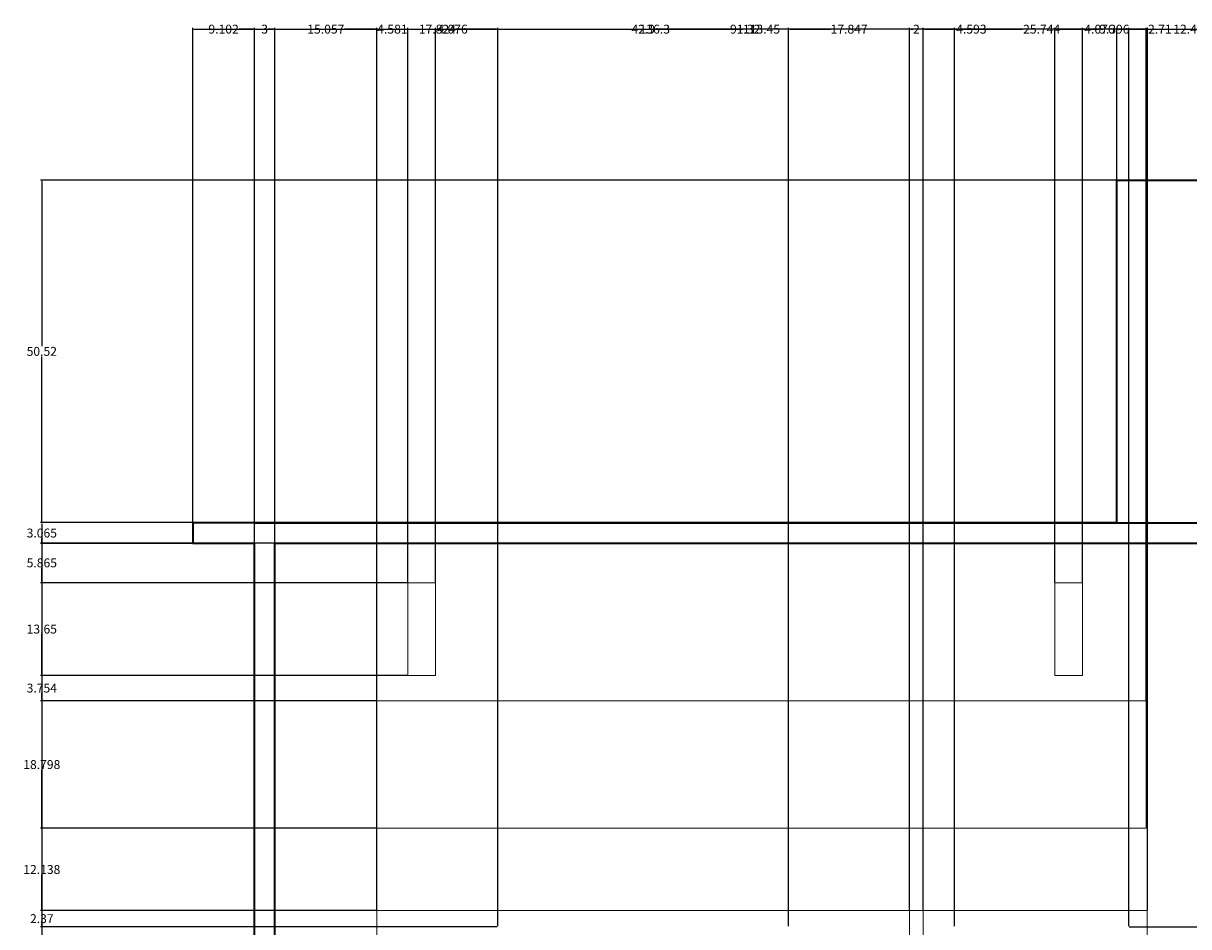
# Model space of a CAD drawing. Units: inches. Extents: x 30 to 515, y 94 to 489.
# Tile 3 of 7: x 30 to 202, y 356 to 489. Entities that reach past the tile are written whole.
import ezdxf

# ---------------------------------------------------------------- set-up
doc = ezdxf.new("R2010")
doc.units = ezdxf.units.IN
doc.header["$MEASUREMENT"] = 0
for name, color, linetype, lineweight in [('A-ANNO-DIMS', 2, 'Continuous', 18), ('A-ELEV', 8, 'Continuous', 18), ('A-FLOR-HRAL', 3, 'Continuous', 18), ('A-ROOF', 1, 'Continuous', 35), ('A-WALL', 7, 'Continuous', 35)]:
    doc.layers.add(name, color=color, linetype=linetype, lineweight=lineweight)
doc.styles.get("Standard").update_dxf_attribs({"font": 'arial.ttf'})
doc.dimstyles.get("Standard").update_dxf_attribs({"dimtxt": 1.3125, "dimasz": 0.18, "dimexe": 0.18, "dimexo": 0.0625, "dimgap": 0.09, "dimtad": 0, "dimtih": 1, "dimtoh": 1, "dimdec": 4, "dimzin": 0, "dimdsep": 46, "dimlunit": 4, "dimtxsty": 'Standard', "dimcen": 0.09, "dimadec": 0, "dimazin": 0, "dimtfac": 1, "dimtdec": 4, "dimtofl": 0, "dimtmove": 0, "dimatfit": 3, "dimfxl": 1, "dimtolj": 1, "dimtzin": 0, "dimarcsym": 0})

# ---------------------------------------------------------------- blocks, each defined once
blk = doc.blocks.new('*D4')
at = {"layer": 'A-ANNO-DIMS', "color": 0, "lineweight": -2, "transparency": 16777216}
for p, q in [((54.91, 415.59), (54.91, 488.48)), ((55.09, 488.3), (120.82, 488.3)), ((191.03, 488.3), (125.31, 488.3)), ((191.21, 466.11), (191.21, 488.48))]:
    blk.add_line(p, q, dxfattribs=at)
at = {"layer": 'A-ANNO-DIMS', "color": 0, "transparency": 16777216}
for points in [[(55.09, 488.33), (55.09, 488.27), (54.91, 488.3)], [(191.03, 488.33), (191.03, 488.27), (191.21, 488.3)]]:
    blk.add_solid(points, dxfattribs=at)
at = {"layer": 'Defpoints', "color": 0, "transparency": 16777216}
for p in [(191.21, 488.3), (191.21, 466.05), (54.91, 415.53)]:
    blk.add_point(p, dxfattribs=at)
at = {"layer": 'A-ANNO-DIMS', "color": 0, "transparency": 16777216, "insert": (123.06, 488.3), "char_height": 1.312, "attachment_point": 5}
blk.add_mtext('\\A1;136.3', dxfattribs=at)
blk = doc.blocks.new('*D5')
at = {"layer": 'A-ANNO-DIMS', "color": 0, "lineweight": -2, "transparency": 16777216}
for p, q in [((191.21, 466.11), (191.21, 488.48)), ((191.39, 488.3), (285.04, 488.3)), ((384.19, 488.3), (290.54, 488.3)), ((384.37, 466.11), (384.37, 488.48))]:
    blk.add_line(p, q, dxfattribs=at)
at = {"layer": 'A-ANNO-DIMS', "color": 0, "transparency": 16777216}
for points in [[(191.39, 488.33), (191.39, 488.27), (191.21, 488.3)], [(384.19, 488.33), (384.19, 488.27), (384.37, 488.3)]]:
    blk.add_solid(points, dxfattribs=at)
at = {"layer": 'Defpoints', "color": 0, "transparency": 16777216}
for p in [(384.37, 488.3), (191.21, 466.05), (384.37, 466.05)]:
    blk.add_point(p, dxfattribs=at)
at = {"layer": 'A-ANNO-DIMS', "color": 0, "transparency": 16777216, "insert": (287.79, 488.3), "char_height": 1.312, "attachment_point": 5}
blk.add_mtext('\\A1;193.16', dxfattribs=at)
blk = doc.blocks.new('*D25')
at = {"layer": 'A-ANNO-DIMS', "color": 0, "lineweight": -2, "transparency": 16777216}
for p, q in [((66.95, 415.53), (32.48, 415.53)), ((32.66, 415.35), (32.66, 342.78)), ((32.66, 268.71), (32.66, 341.28)), ((66.95, 268.53), (32.48, 268.53))]:
    blk.add_line(p, q, dxfattribs=at)
at = {"layer": 'A-ANNO-DIMS', "color": 0, "transparency": 16777216}
for points in [[(32.63, 415.35), (32.69, 415.35), (32.66, 415.53)], [(32.63, 268.71), (32.69, 268.71), (32.66, 268.53)]]:
    blk.add_solid(points, dxfattribs=at)
at = {"layer": 'Defpoints', "color": 0, "transparency": 16777216}
for p in [(32.66, 415.53), (67.02, 415.53), (67.02, 268.53)]:
    blk.add_point(p, dxfattribs=at)
at = {"layer": 'A-ANNO-DIMS', "color": 0, "transparency": 16777216, "insert": (32.66, 342.03), "char_height": 1.312, "attachment_point": 5}
blk.add_mtext('\\A1;147', dxfattribs=at)
blk = doc.blocks.new('*D26')
at = {"layer": 'A-ANNO-DIMS', "color": 0, "lineweight": -2, "transparency": 16777216}
for p, q in [((54.85, 415.53), (32.48, 415.53)), ((32.66, 415.35), (32.66, 414.76)), ((32.66, 412.64), (32.66, 413.23)), ((54.85, 412.46), (32.48, 412.46))]:
    blk.add_line(p, q, dxfattribs=at)
at = {"layer": 'A-ANNO-DIMS', "color": 0, "transparency": 16777216}
for points in [[(32.63, 415.35), (32.69, 415.35), (32.66, 415.53)], [(32.63, 412.64), (32.69, 412.64), (32.66, 412.46)]]:
    blk.add_solid(points, dxfattribs=at)
at = {"layer": 'Defpoints', "color": 0, "transparency": 16777216}
for p in [(32.66, 415.53), (54.91, 415.53), (54.91, 412.46)]:
    blk.add_point(p, dxfattribs=at)
at = {"layer": 'A-ANNO-DIMS', "color": 0, "transparency": 16777216, "insert": (32.66, 414), "char_height": 1.312, "attachment_point": 5}
blk.add_mtext('\\A1;3.065', dxfattribs=at)
blk = doc.blocks.new('*D27')
at = {"layer": 'A-ANNO-DIMS', "color": 0, "lineweight": -2, "transparency": 16777216}
for p, q in [((191.15, 466.05), (32.48, 466.05)), ((32.66, 465.87), (32.66, 441.55)), ((32.66, 415.71), (32.66, 440.03)), ((191.15, 415.53), (32.48, 415.53))]:
    blk.add_line(p, q, dxfattribs=at)
at = {"layer": 'A-ANNO-DIMS', "color": 0, "transparency": 16777216}
for points in [[(32.63, 465.87), (32.69, 465.87), (32.66, 466.05)], [(32.63, 415.71), (32.69, 415.71), (32.66, 415.53)]]:
    blk.add_solid(points, dxfattribs=at)
at = {"layer": 'Defpoints', "color": 0, "transparency": 16777216}
for p in [(32.66, 466.05), (191.21, 466.05), (191.21, 415.53)]:
    blk.add_point(p, dxfattribs=at)
at = {"layer": 'A-ANNO-DIMS', "color": 0, "transparency": 16777216, "insert": (32.66, 440.79), "char_height": 1.312, "attachment_point": 5}
blk.add_mtext('\\A1;50.52', dxfattribs=at)
blk = doc.blocks.new('*D31')
at = {"layer": 'A-ANNO-DIMS', "color": 0, "lineweight": -2, "transparency": 16777216}
for p, q in [((54.91, 412.53), (54.91, 488.48)), ((55.09, 488.3), (57.17, 488.3)), ((63.84, 488.3), (61.76, 488.3)), ((64.02, 412.57), (64.02, 488.48))]:
    blk.add_line(p, q, dxfattribs=at)
at = {"layer": 'A-ANNO-DIMS', "color": 0, "transparency": 16777216}
for points in [[(55.09, 488.33), (55.09, 488.27), (54.91, 488.3)], [(63.84, 488.33), (63.84, 488.27), (64.02, 488.3)]]:
    blk.add_solid(points, dxfattribs=at)
at = {"layer": 'Defpoints', "color": 0, "transparency": 16777216}
for p in [(64.02, 488.3), (64.02, 412.51), (54.91, 412.46)]:
    blk.add_point(p, dxfattribs=at)
at = {"layer": 'A-ANNO-DIMS', "color": 0, "transparency": 16777216, "insert": (59.47, 488.3), "char_height": 1.312, "attachment_point": 5}
blk.add_mtext('\\A1;9.102', dxfattribs=at)
blk = doc.blocks.new('*D32')
at = {"layer": 'A-ANNO-DIMS', "color": 0, "lineweight": -2, "transparency": 16777216}
for p, q in [((64.02, 412.57), (64.02, 488.48)), ((64.2, 488.3), (65, 488.3)), ((66.84, 488.3), (66.04, 488.3)), ((67.02, 412.59), (67.02, 488.48))]:
    blk.add_line(p, q, dxfattribs=at)
at = {"layer": 'A-ANNO-DIMS', "color": 0, "transparency": 16777216}
for points in [[(64.2, 488.33), (64.2, 488.27), (64.02, 488.3)], [(66.84, 488.33), (66.84, 488.27), (67.02, 488.3)]]:
    blk.add_solid(points, dxfattribs=at)
at = {"layer": 'Defpoints', "color": 0, "transparency": 16777216}
for p in [(67.02, 488.3), (64.02, 412.51), (67.02, 412.53)]:
    blk.add_point(p, dxfattribs=at)
at = {"layer": 'A-ANNO-DIMS', "color": 0, "transparency": 16777216, "insert": (65.52, 488.3), "char_height": 1.312, "attachment_point": 5}
blk.add_mtext('\\A1;3', dxfattribs=at)
blk = doc.blocks.new('*D33')
at = {"layer": 'A-ANNO-DIMS', "color": 0, "lineweight": -2, "transparency": 16777216}
for p, q in [((67.02, 412.59), (67.02, 488.48)), ((67.2, 488.3), (71.79, 488.3)), ((81.89, 488.3), (77.3, 488.3)), ((82.07, 389.32), (82.07, 488.48))]:
    blk.add_line(p, q, dxfattribs=at)
at = {"layer": 'A-ANNO-DIMS', "color": 0, "transparency": 16777216}
for points in [[(67.2, 488.33), (67.2, 488.27), (67.02, 488.3)], [(81.89, 488.33), (81.89, 488.27), (82.07, 488.3)]]:
    blk.add_solid(points, dxfattribs=at)
at = {"layer": 'Defpoints', "color": 0, "transparency": 16777216}
for p in [(82.07, 488.3), (67.02, 412.53), (82.07, 389.26)]:
    blk.add_point(p, dxfattribs=at)
at = {"layer": 'A-ANNO-DIMS', "color": 0, "transparency": 16777216, "insert": (74.55, 488.3), "char_height": 1.312, "attachment_point": 5}
blk.add_mtext('\\A1;15.057', dxfattribs=at)
blk = doc.blocks.new('*D34')
at = {"layer": 'A-ANNO-DIMS', "color": 0, "lineweight": -2, "transparency": 16777216}
for p, q in [((81.893567, 488.300291), (81.713567, 488.300291)), ((82.073567, 389.322756), (82.073567, 488.480291)), ((86.654989, 406.725431), (86.654989, 488.480291)), ((86.834989, 488.300291), (87.014989, 488.300291))]:
    blk.add_line(p, q, dxfattribs=at)
at = {"layer": 'A-ANNO-DIMS', "color": 0, "transparency": 16777216}
for points in [[(81.893567, 488.330291), (81.893567, 488.270291), (82.073567, 488.300291)], [(86.834989, 488.330291), (86.834989, 488.270291), (86.654989, 488.300291)]]:
    blk.add_solid(points, dxfattribs=at)
at = {"layer": 'Defpoints', "color": 0, "transparency": 16777216}
for p in [(86.654989, 488.300291), (86.654989, 406.662931), (82.073567, 389.260256)]:
    blk.add_point(p, dxfattribs=at)
at = {"layer": 'A-ANNO-DIMS', "color": 0, "transparency": 16777216, "insert": (84.364278, 488.300291), "char_height": 1.3125, "attachment_point": 5}
blk.add_mtext('\\A1;4.581', dxfattribs=at)
blk = doc.blocks.new('*D35')
at = {"layer": 'A-ANNO-DIMS', "color": 0, "lineweight": -2, "transparency": 16777216}
for p, q in [((86.65, 406.73), (86.65, 488.48)), ((86.83, 488.3), (90.55, 488.3)), ((90.73, 406.73), (90.73, 488.48)), ((90.73, 488.3), (90.91, 488.3))]:
    blk.add_line(p, q, dxfattribs=at)
at = {"layer": 'A-ANNO-DIMS', "color": 0, "transparency": 16777216}
for points in [[(86.83, 488.33), (86.83, 488.27), (86.65, 488.3)], [(90.55, 488.33), (90.55, 488.27), (90.73, 488.3)]]:
    blk.add_solid(points, dxfattribs=at)
at = {"layer": 'Defpoints', "color": 0, "transparency": 16777216}
for p in [(90.73, 488.3), (86.65, 406.66), (90.73, 406.66)]:
    blk.add_point(p, dxfattribs=at)
at = {"layer": 'A-ANNO-DIMS', "color": 0, "transparency": 16777216, "insert": (93.24, 488.3), "char_height": 1.312, "attachment_point": 5}
blk.add_mtext('\\A1;4.076', dxfattribs=at)
blk = doc.blocks.new('*D36')
at = {"layer": 'A-ANNO-DIMS', "color": 0, "lineweight": -2, "transparency": 16777216}
for p, q in [((90.73, 406.73), (90.73, 488.48)), ((90.91, 488.3), (134.09, 488.3)), ((181.87, 488.3), (138.69, 488.3)), ((182.05, 406.73), (182.05, 488.48))]:
    blk.add_line(p, q, dxfattribs=at)
at = {"layer": 'A-ANNO-DIMS', "color": 0, "transparency": 16777216}
for points in [[(90.91, 488.33), (90.91, 488.27), (90.73, 488.3)], [(181.87, 488.33), (181.87, 488.27), (182.05, 488.3)]]:
    blk.add_solid(points, dxfattribs=at)
at = {"layer": 'Defpoints', "color": 0, "transparency": 16777216}
for p in [(182.05, 488.3), (90.73, 406.66), (182.05, 406.66)]:
    blk.add_point(p, dxfattribs=at)
at = {"layer": 'A-ANNO-DIMS', "color": 0, "transparency": 16777216, "insert": (136.39, 488.3), "char_height": 1.312, "attachment_point": 5}
blk.add_mtext('\\A1;91.32', dxfattribs=at)
blk = doc.blocks.new('*D37')
at = {"layer": 'A-ANNO-DIMS', "color": 0, "lineweight": -2, "transparency": 16777216}
for p, q in [((182.05, 406.73), (182.05, 488.48)), ((182.23, 488.3), (185.95, 488.3)), ((186.13, 406.73), (186.13, 488.48)), ((186.13, 488.3), (186.31, 488.3))]:
    blk.add_line(p, q, dxfattribs=at)
at = {"layer": 'A-ANNO-DIMS', "color": 0, "transparency": 16777216}
for points in [[(182.23, 488.33), (182.23, 488.27), (182.05, 488.3)], [(185.95, 488.33), (185.95, 488.27), (186.13, 488.3)]]:
    blk.add_solid(points, dxfattribs=at)
at = {"layer": 'Defpoints', "color": 0, "transparency": 16777216}
for p in [(186.13, 488.3), (182.05, 406.66), (186.13, 406.66)]:
    blk.add_point(p, dxfattribs=at)
at = {"layer": 'A-ANNO-DIMS', "color": 0, "transparency": 16777216, "insert": (188.64, 488.3), "char_height": 1.312, "attachment_point": 5}
blk.add_mtext('\\A1;4.076', dxfattribs=at)
blk = doc.blocks.new('*D38')
at = {"layer": 'A-ANNO-DIMS', "color": 0, "lineweight": -2, "transparency": 16777216}
for p, q in [((186.13, 406.73), (186.13, 488.48)), ((186.31, 488.3), (188.52, 488.3)), ((195.35, 488.3), (193.13, 488.3)), ((195.53, 389.32), (195.53, 488.48))]:
    blk.add_line(p, q, dxfattribs=at)
at = {"layer": 'A-ANNO-DIMS', "color": 0, "transparency": 16777216}
for points in [[(186.31, 488.33), (186.31, 488.27), (186.13, 488.3)], [(195.35, 488.33), (195.35, 488.27), (195.53, 488.3)]]:
    blk.add_solid(points, dxfattribs=at)
at = {"layer": 'Defpoints', "color": 0, "transparency": 16777216}
for p in [(195.53, 488.3), (186.13, 406.66), (195.53, 389.26)]:
    blk.add_point(p, dxfattribs=at)
at = {"layer": 'A-ANNO-DIMS', "color": 0, "transparency": 16777216, "insert": (190.83, 488.3), "char_height": 1.312, "attachment_point": 5}
blk.add_mtext('\\A1;9.396', dxfattribs=at)
blk = doc.blocks.new('*D39')
at = {"layer": 'A-ANNO-DIMS', "color": 0, "lineweight": -2, "transparency": 16777216}
for p, q in [((195.53, 389.32), (195.53, 488.48)), ((195.71, 488.3), (199.51, 488.3)), ((207.81, 488.3), (204, 488.3)), ((207.99, 412.59), (207.99, 488.48))]:
    blk.add_line(p, q, dxfattribs=at)
at = {"layer": 'A-ANNO-DIMS', "color": 0, "transparency": 16777216}
for points in [[(195.71, 488.33), (195.71, 488.27), (195.53, 488.3)], [(207.81, 488.33), (207.81, 488.27), (207.99, 488.3)]]:
    blk.add_solid(points, dxfattribs=at)
at = {"layer": 'Defpoints', "color": 0, "transparency": 16777216}
for p in [(207.99, 488.3), (207.99, 412.53), (195.53, 389.26)]:
    blk.add_point(p, dxfattribs=at)
at = {"layer": 'A-ANNO-DIMS', "color": 0, "transparency": 16777216, "insert": (201.76, 488.3), "char_height": 1.312, "attachment_point": 5}
blk.add_mtext('\\A1;12.46', dxfattribs=at)
blk = doc.blocks.new('*D41')
at = {"layer": 'A-ANNO-DIMS', "color": 0, "lineweight": -2, "transparency": 16777216}
for p, q in [((82.07, 389.32), (82.07, 488.48)), ((82.25, 488.3), (136.04, 488.3)), ((195.35, 488.3), (141.56, 488.3)), ((195.53, 389.32), (195.53, 488.48))]:
    blk.add_line(p, q, dxfattribs=at)
at = {"layer": 'A-ANNO-DIMS', "color": 0, "transparency": 16777216}
for points in [[(82.25, 488.33), (82.25, 488.27), (82.07, 488.3)], [(195.35, 488.33), (195.35, 488.27), (195.53, 488.3)]]:
    blk.add_solid(points, dxfattribs=at)
at = {"layer": 'Defpoints', "color": 0, "transparency": 16777216}
for p in [(195.53, 488.3), (82.07, 389.26), (195.53, 389.26)]:
    blk.add_point(p, dxfattribs=at)
at = {"layer": 'A-ANNO-DIMS', "color": 0, "transparency": 16777216, "insert": (138.8, 488.3), "char_height": 1.312, "attachment_point": 5}
blk.add_mtext('\\A1;113.45', dxfattribs=at)
blk = doc.blocks.new('*D42')
at = {"layer": 'A-ANNO-DIMS', "color": 0, "lineweight": -2, "transparency": 16777216}
for p, q in [((82.07, 358.39), (82.07, 488.48)), ((82.25, 488.3), (88.24, 488.3)), ((99.72, 488.3), (93.74, 488.3)), ((99.9, 356.02), (99.9, 488.48))]:
    blk.add_line(p, q, dxfattribs=at)
at = {"layer": 'A-ANNO-DIMS', "color": 0, "transparency": 16777216}
for points in [[(82.25, 488.33), (82.25, 488.27), (82.07, 488.3)], [(99.72, 488.33), (99.72, 488.27), (99.9, 488.3)]]:
    blk.add_solid(points, dxfattribs=at)
at = {"layer": 'Defpoints', "color": 0, "transparency": 16777216}
for p in [(99.9, 488.3), (82.07, 358.32), (99.9, 355.95)]:
    blk.add_point(p, dxfattribs=at)
at = {"layer": 'A-ANNO-DIMS', "color": 0, "transparency": 16777216, "insert": (90.99, 488.3), "char_height": 1.312, "attachment_point": 5}
blk.add_mtext('\\A1;17.824', dxfattribs=at)
blk = doc.blocks.new('*D43')
at = {"layer": 'A-ANNO-DIMS', "color": 0, "lineweight": -2, "transparency": 16777216}
for p, q in [((99.9, 356.02), (99.9, 488.48)), ((100.08, 488.3), (119.52, 488.3)), ((142.62, 488.3), (123.17, 488.3)), ((142.8, 356.02), (142.8, 488.48))]:
    blk.add_line(p, q, dxfattribs=at)
at = {"layer": 'A-ANNO-DIMS', "color": 0, "transparency": 16777216}
for points in [[(100.08, 488.33), (100.08, 488.27), (99.9, 488.3)], [(142.62, 488.33), (142.62, 488.27), (142.8, 488.3)]]:
    blk.add_solid(points, dxfattribs=at)
at = {"layer": 'Defpoints', "color": 0, "transparency": 16777216}
for p in [(142.8, 488.3), (99.9, 355.95), (142.8, 355.95)]:
    blk.add_point(p, dxfattribs=at)
at = {"layer": 'A-ANNO-DIMS', "color": 0, "transparency": 16777216, "insert": (121.35, 488.3), "char_height": 1.312, "attachment_point": 5}
blk.add_mtext('\\A1;42.9', dxfattribs=at)
blk = doc.blocks.new('*D44')
at = {"layer": 'A-ANNO-DIMS', "color": 0, "lineweight": -2, "transparency": 16777216}
for p, q in [((142.8, 356.02), (142.8, 488.48)), ((142.98, 488.3), (148.97, 488.3)), ((160.46, 488.3), (154.47, 488.3)), ((160.64, 358.39), (160.64, 488.48))]:
    blk.add_line(p, q, dxfattribs=at)
at = {"layer": 'A-ANNO-DIMS', "color": 0, "transparency": 16777216}
for points in [[(142.98, 488.33), (142.98, 488.27), (142.8, 488.3)], [(160.46, 488.33), (160.46, 488.27), (160.64, 488.3)]]:
    blk.add_solid(points, dxfattribs=at)
at = {"layer": 'Defpoints', "color": 0, "transparency": 16777216}
for p in [(160.64, 488.3), (160.64, 358.32), (142.8, 355.95)]:
    blk.add_point(p, dxfattribs=at)
at = {"layer": 'A-ANNO-DIMS', "color": 0, "transparency": 16777216, "insert": (151.72, 488.3), "char_height": 1.312, "attachment_point": 5}
blk.add_mtext('\\A1;17.847', dxfattribs=at)
blk = doc.blocks.new('*D45')
at = {"layer": 'A-ANNO-DIMS', "color": 0, "lineweight": -2, "transparency": 16777216}
for p, q in [((160.64, 358.39), (160.64, 488.48)), ((160.82, 488.3), (161.12, 488.3)), ((162.46, 488.3), (162.17, 488.3)), ((162.64, 358.39), (162.64, 488.48))]:
    blk.add_line(p, q, dxfattribs=at)
at = {"layer": 'A-ANNO-DIMS', "color": 0, "transparency": 16777216}
for points in [[(160.82, 488.33), (160.82, 488.27), (160.64, 488.3)], [(162.46, 488.33), (162.46, 488.27), (162.64, 488.3)]]:
    blk.add_solid(points, dxfattribs=at)
at = {"layer": 'Defpoints', "color": 0, "transparency": 16777216}
for p in [(162.64, 488.3), (160.64, 358.32), (162.64, 358.32)]:
    blk.add_point(p, dxfattribs=at)
at = {"layer": 'A-ANNO-DIMS', "color": 0, "transparency": 16777216, "insert": (161.64, 488.3), "char_height": 1.312, "attachment_point": 5}
blk.add_mtext('\\A1;2', dxfattribs=at)
blk = doc.blocks.new('*D46')
at = {"layer": 'A-ANNO-DIMS', "color": 0, "lineweight": -2, "transparency": 16777216}
for p, q in [((162.64, 358.39), (162.64, 488.48)), ((162.82, 488.3), (167.06, 488.3)), ((167.24, 356.02), (167.24, 488.48)), ((167.24, 488.3), (167.42, 488.3))]:
    blk.add_line(p, q, dxfattribs=at)
at = {"layer": 'A-ANNO-DIMS', "color": 0, "transparency": 16777216}
for points in [[(162.82, 488.33), (162.82, 488.27), (162.64, 488.3)], [(167.06, 488.33), (167.06, 488.27), (167.24, 488.3)]]:
    blk.add_solid(points, dxfattribs=at)
at = {"layer": 'Defpoints', "color": 0, "transparency": 16777216}
for p in [(167.24, 488.3), (162.64, 358.32), (167.24, 355.95)]:
    blk.add_point(p, dxfattribs=at)
at = {"layer": 'A-ANNO-DIMS', "color": 0, "transparency": 16777216, "insert": (169.75, 488.3), "char_height": 1.312, "attachment_point": 5}
blk.add_mtext('\\A1;4.593', dxfattribs=at)
blk = doc.blocks.new('*D47')
at = {"layer": 'A-ANNO-DIMS', "color": 0, "lineweight": -2, "transparency": 16777216}
for p, q in [((167.24, 356.02), (167.24, 488.48)), ((167.42, 488.3), (177.29, 488.3)), ((192.8, 488.3), (182.93, 488.3)), ((192.98, 356.02), (192.98, 488.48))]:
    blk.add_line(p, q, dxfattribs=at)
at = {"layer": 'A-ANNO-DIMS', "color": 0, "transparency": 16777216}
for points in [[(167.42, 488.33), (167.42, 488.27), (167.24, 488.3)], [(192.8, 488.33), (192.8, 488.27), (192.98, 488.3)]]:
    blk.add_solid(points, dxfattribs=at)
at = {"layer": 'Defpoints', "color": 0, "transparency": 16777216}
for p in [(192.98, 488.3), (167.24, 355.95), (192.98, 355.95)]:
    blk.add_point(p, dxfattribs=at)
at = {"layer": 'A-ANNO-DIMS', "color": 0, "transparency": 16777216, "insert": (180.11, 488.3), "char_height": 1.312, "attachment_point": 5}
blk.add_mtext('\\A1;25.744', dxfattribs=at)
blk = doc.blocks.new('*D48')
at = {"layer": 'A-ANNO-DIMS', "color": 0, "lineweight": -2, "transparency": 16777216}
for p, q in [((192.98, 356.02), (192.98, 488.48)), ((193.16, 488.3), (195.52, 488.3)), ((195.7, 358.39), (195.7, 488.48)), ((195.7, 488.3), (195.88, 488.3))]:
    blk.add_line(p, q, dxfattribs=at)
at = {"layer": 'A-ANNO-DIMS', "color": 0, "transparency": 16777216}
for points in [[(193.16, 488.33), (193.16, 488.27), (192.98, 488.3)], [(195.52, 488.33), (195.52, 488.27), (195.7, 488.3)]]:
    blk.add_solid(points, dxfattribs=at)
at = {"layer": 'Defpoints', "color": 0, "transparency": 16777216}
for p in [(195.7, 488.3), (195.7, 358.32), (192.98, 355.95)]:
    blk.add_point(p, dxfattribs=at)
at = {"layer": 'A-ANNO-DIMS', "color": 0, "transparency": 16777216, "insert": (197.55, 488.3), "char_height": 1.312, "attachment_point": 5}
blk.add_mtext('\\A1;2.71', dxfattribs=at)
blk = doc.blocks.new('*D52')
at = {"layer": 'A-ANNO-DIMS', "color": 0, "lineweight": -2, "transparency": 16777216}
for p, q in [((99.83, 355.95), (32.48, 355.95)), ((32.66, 355.77), (32.66, 343.38)), ((32.66, 329.46), (32.66, 341.86)), ((99.83, 329.28), (32.48, 329.28))]:
    blk.add_line(p, q, dxfattribs=at)
at = {"layer": 'A-ANNO-DIMS', "color": 0, "transparency": 16777216}
for points in [[(32.63, 355.77), (32.69, 355.77), (32.66, 355.95)], [(32.63, 329.46), (32.69, 329.46), (32.66, 329.28)]]:
    blk.add_solid(points, dxfattribs=at)
at = {"layer": 'Defpoints', "color": 0, "transparency": 16777216}
for p in [(32.66, 355.95), (99.9, 355.95), (99.9, 329.28)]:
    blk.add_point(p, dxfattribs=at)
at = {"layer": 'A-ANNO-DIMS', "color": 0, "transparency": 16777216, "insert": (32.66, 342.62), "char_height": 1.312, "attachment_point": 5}
blk.add_mtext('\\A1;26.675', dxfattribs=at)
blk = doc.blocks.new('*D53')
at = {"layer": 'A-ANNO-DIMS', "color": 0, "lineweight": -2, "transparency": 16777216}
for p, q in [((82.01, 358.32), (32.48, 358.32)), ((32.66, 358.14), (32.66, 357.9)), ((99.83, 355.95), (32.48, 355.95)), ((32.66, 356.13), (32.66, 356.38))]:
    blk.add_line(p, q, dxfattribs=at)
at = {"layer": 'A-ANNO-DIMS', "color": 0, "transparency": 16777216}
for points in [[(32.63, 358.14), (32.69, 358.14), (32.66, 358.32)], [(32.63, 356.13), (32.69, 356.13), (32.66, 355.95)]]:
    blk.add_solid(points, dxfattribs=at)
at = {"layer": 'Defpoints', "color": 0, "transparency": 16777216}
for p in [(32.66, 358.32), (82.07, 358.32), (99.9, 355.95)]:
    blk.add_point(p, dxfattribs=at)
at = {"layer": 'A-ANNO-DIMS', "color": 0, "transparency": 16777216, "insert": (32.66, 357.14), "char_height": 1.312, "attachment_point": 5}
blk.add_mtext('\\A1;2.37', dxfattribs=at)
blk = doc.blocks.new('*D54')
at = {"layer": 'A-ANNO-DIMS', "color": 0, "lineweight": -2, "transparency": 16777216}
for p, q in [((82.01, 370.46), (32.48, 370.46)), ((32.66, 370.28), (32.66, 365.15)), ((32.66, 358.5), (32.66, 363.63)), ((82.01, 358.32), (32.48, 358.32))]:
    blk.add_line(p, q, dxfattribs=at)
at = {"layer": 'A-ANNO-DIMS', "color": 0, "transparency": 16777216}
for points in [[(32.63, 370.28), (32.69, 370.28), (32.66, 370.46)], [(32.63, 358.5), (32.69, 358.5), (32.66, 358.32)]]:
    blk.add_solid(points, dxfattribs=at)
at = {"layer": 'Defpoints', "color": 0, "transparency": 16777216}
for p in [(32.66, 370.46), (82.07, 370.46), (82.07, 358.32)]:
    blk.add_point(p, dxfattribs=at)
at = {"layer": 'A-ANNO-DIMS', "color": 0, "transparency": 16777216, "insert": (32.66, 364.39), "char_height": 1.312, "attachment_point": 5}
blk.add_mtext('\\A1;12.138', dxfattribs=at)
blk = doc.blocks.new('*D55')
at = {"layer": 'A-ANNO-DIMS', "color": 0, "lineweight": -2, "transparency": 16777216}
for p, q in [((82.01, 389.26), (32.48, 389.26)), ((32.66, 389.08), (32.66, 380.62)), ((32.66, 370.64), (32.66, 379.1)), ((82.01, 370.46), (32.48, 370.46))]:
    blk.add_line(p, q, dxfattribs=at)
at = {"layer": 'A-ANNO-DIMS', "color": 0, "transparency": 16777216}
for points in [[(32.63, 389.08), (32.69, 389.08), (32.66, 389.26)], [(32.63, 370.64), (32.69, 370.64), (32.66, 370.46)]]:
    blk.add_solid(points, dxfattribs=at)
at = {"layer": 'Defpoints', "color": 0, "transparency": 16777216}
for p in [(32.66, 389.26), (82.07, 389.26), (82.07, 370.46)]:
    blk.add_point(p, dxfattribs=at)
at = {"layer": 'A-ANNO-DIMS', "color": 0, "transparency": 16777216, "insert": (32.66, 379.86), "char_height": 1.312, "attachment_point": 5}
blk.add_mtext('\\A1;18.798', dxfattribs=at)
blk = doc.blocks.new('*D56')
at = {"layer": 'A-ANNO-DIMS', "color": 0, "lineweight": -2, "transparency": 16777216}
for p, q in [((86.59, 393.01), (32.48, 393.01)), ((32.66, 392.83), (32.66, 391.9)), ((32.66, 389.44), (32.66, 390.38)), ((82.01, 389.26), (32.48, 389.26))]:
    blk.add_line(p, q, dxfattribs=at)
at = {"layer": 'A-ANNO-DIMS', "color": 0, "transparency": 16777216}
for points in [[(32.63, 392.83), (32.69, 392.83), (32.66, 393.01)], [(32.63, 389.44), (32.69, 389.44), (32.66, 389.26)]]:
    blk.add_solid(points, dxfattribs=at)
at = {"layer": 'Defpoints', "color": 0, "transparency": 16777216}
for p in [(32.66, 393.01), (86.65, 393.01), (82.07, 389.26)]:
    blk.add_point(p, dxfattribs=at)
at = {"layer": 'A-ANNO-DIMS', "color": 0, "transparency": 16777216, "insert": (32.66, 391.14), "char_height": 1.312, "attachment_point": 5}
blk.add_mtext('\\A1;3.754', dxfattribs=at)
blk = doc.blocks.new('*D57')
at = {"layer": 'A-ANNO-DIMS', "color": 0, "lineweight": -2, "transparency": 16777216}
for p, q in [((86.59, 406.66), (32.48, 406.66)), ((32.66, 406.48), (32.66, 400.6)), ((32.66, 393.19), (32.66, 399.08)), ((86.59, 393.01), (32.48, 393.01))]:
    blk.add_line(p, q, dxfattribs=at)
at = {"layer": 'A-ANNO-DIMS', "color": 0, "transparency": 16777216}
for points in [[(32.63, 406.48), (32.69, 406.48), (32.66, 406.66)], [(32.63, 393.19), (32.69, 393.19), (32.66, 393.01)]]:
    blk.add_solid(points, dxfattribs=at)
at = {"layer": 'Defpoints', "color": 0, "transparency": 16777216}
for p in [(32.66, 406.66), (86.65, 406.66), (86.65, 393.01)]:
    blk.add_point(p, dxfattribs=at)
at = {"layer": 'A-ANNO-DIMS', "color": 0, "transparency": 16777216, "insert": (32.66, 399.84), "char_height": 1.312, "attachment_point": 5}
blk.add_mtext('\\A1;13.65', dxfattribs=at)
blk = doc.blocks.new('*D58')
at = {"layer": 'A-ANNO-DIMS', "color": 0, "lineweight": -2, "transparency": 16777216}
for p, q in [((66.95, 412.53), (32.48, 412.53)), ((32.66, 412.35), (32.66, 410.36)), ((32.66, 406.84), (32.66, 408.84)), ((86.59, 406.66), (32.48, 406.66))]:
    blk.add_line(p, q, dxfattribs=at)
at = {"layer": 'A-ANNO-DIMS', "color": 0, "transparency": 16777216}
for points in [[(32.63, 412.35), (32.69, 412.35), (32.66, 412.53)], [(32.63, 406.84), (32.69, 406.84), (32.66, 406.66)]]:
    blk.add_solid(points, dxfattribs=at)
at = {"layer": 'Defpoints', "color": 0, "transparency": 16777216}
for p in [(32.66, 412.53), (67.02, 412.53), (86.65, 406.66)]:
    blk.add_point(p, dxfattribs=at)
at = {"layer": 'A-ANNO-DIMS', "color": 0, "transparency": 16777216, "insert": (32.66, 409.6), "char_height": 1.312, "attachment_point": 5}
blk.add_mtext('\\A1;5.865', dxfattribs=at)
blk = doc.blocks.new('*D61')
at = {"layer": 'A-ANNO-DIMS', "color": 0, "lineweight": -2, "transparency": 16777216}
for p, q in [((193.04, 355.95), (512.17, 355.95)), ((511.99, 355.77), (511.99, 339.15)), ((511.99, 321.01), (511.99, 337.63)), ((191.31, 320.83), (512.17, 320.83))]:
    blk.add_line(p, q, dxfattribs=at)
at = {"layer": 'A-ANNO-DIMS', "color": 0, "transparency": 16777216}
for points in [[(511.96, 355.77), (512.02, 355.77), (511.99, 355.95)], [(511.96, 321.01), (512.02, 321.01), (511.99, 320.83)]]:
    blk.add_solid(points, dxfattribs=at)
at = {"layer": 'Defpoints', "color": 0, "transparency": 16777216}
for p in [(192.98, 355.95), (511.99, 355.95), (191.25, 320.83)]:
    blk.add_point(p, dxfattribs=at)
at = {"layer": 'A-ANNO-DIMS', "color": 0, "transparency": 16777216, "insert": (511.99, 338.39), "char_height": 1.312, "attachment_point": 5}
blk.add_mtext('\\A1;35.13', dxfattribs=at)

msp = doc.modelspace()

# ---------------------------------------------------------------- linework, layer by layer
at = {"layer": 'A-ELEV'}
for points in [[(86.655, 406.6629), (90.7309, 406.6629), (90.7309, 393.0141), (86.655, 393.0141)], [(182.053, 406.6629), (186.1289, 406.6629), (186.1289, 393.0141), (182.053, 393.0141)], [(82.0736, 370.4623), (195.5251, 370.4623), (195.5251, 389.2603), (82.0736, 389.2603)]]:
    msp.add_lwpolyline(points, close=True, dxfattribs=at)
at = {"layer": 'A-FLOR-HRAL'}
for p, q in [((160.6442, 358.3247), (160.6442, 295.0176)), ((162.6442, 358.3247), (162.6442, 295.0176))]:
    msp.add_line(p, q, dxfattribs=at)
msp.add_lwpolyline([(82.0736, 358.3247), (195.6952, 358.3247), (195.6952, 295.0176), (82.0736, 295.0176)], close=True, dxfattribs=at)
at = {"layer": 'A-ROOF'}
for p, q in [((191.2145, 415.5281), (191.2145, 466.0503)), ((191.2145, 466.0503), (286.8264, 466.0503))]:
    msp.add_line(p, q, dxfattribs=at)
at = {"layer": 'A-WALL'}
for p, q in [((64.017, 415.5281), (54.9147, 415.5281)), ((54.9147, 415.5281), (54.9147, 412.4629)), ((64.017, 415.5281), (67.017, 415.5281)), ((67.017, 415.5281), (448.0511, 415.5281)), ((54.9147, 412.4629), (64.017, 412.5119)), ((64.017, 268.5281), (64.017, 412.5281)), ((67.017, 268.5281), (67.017, 412.5281)), ((67.017, 412.5281), (207.9863, 412.5281))]:
    msp.add_line(p, q, dxfattribs=at)

# ---------------------------------------------------------------- dimensions: what is measured, and where the dimension line sits
at = {"layer": 'A-ANNO-DIMS'}
for base, p1, p2, override, picture, middle in [((191.2145, 488.3003), (54.9147, 415.5281), (191.2145, 466.0503), {"dimdec": 1, "dimlfac": 1, "dimrnd": 0, "dimzin": 0, "dimdsep": 46, "dimlunit": 2}, '*D4', (123.0646, 488.3003)), ((64.017, 488.3003), (54.9147, 412.4629), (64.017, 412.5119), {"dimdec": 3, "dimlfac": 1, "dimrnd": 0, "dimzin": 0, "dimdsep": 46, "dimlunit": 2}, '*D31', (59.4659, 488.3003)), ((67.017, 488.3003), (64.017, 412.5119), (67.017, 412.5281), {"dimdec": 0, "dimlfac": 1, "dimrnd": 0, "dimzin": 0, "dimdsep": 46, "dimlunit": 2}, '*D32', (65.517, 488.3003)), ((82.0736, 488.3003), (67.017, 412.5281), (82.0736, 389.2603), {"dimdec": 3, "dimlfac": 1, "dimrnd": 0, "dimzin": 0, "dimdsep": 46, "dimlunit": 2}, '*D33', (74.5453, 488.3003)), ((86.655, 488.3003), (82.0736, 389.2603), (86.655, 406.6629), {"dimdec": 3, "dimlfac": 1, "dimrnd": 0, "dimzin": 0, "dimdsep": 46, "dimlunit": 2}, '*D34', (84.3643, 488.3003)), ((195.5251, 488.3003), (82.0736, 389.2603), (195.5251, 389.2603), {"dimdec": 2, "dimlfac": 1, "dimrnd": 0, "dimzin": 0, "dimdsep": 46, "dimlunit": 2}, '*D41', (138.7993, 488.3003)), ((99.8974, 488.3003), (82.0736, 358.3247), (99.8974, 355.9547), {"dimdec": 3, "dimlfac": 1, "dimrnd": 0, "dimzin": 0, "dimdsep": 46, "dimlunit": 2}, '*D42', (90.9855, 488.3003)), ((90.7309, 488.3003), (86.655, 406.6629), (90.7309, 406.6629), {"dimdec": 3, "dimlfac": 1, "dimrnd": 0, "dimzin": 0, "dimdsep": 46, "dimlunit": 2}, '*D35', (93.2414, 488.3003)), ((182.053, 488.3003), (90.7309, 406.6629), (182.053, 406.6629), {"dimdec": 2, "dimlfac": 1, "dimrnd": 0, "dimzin": 0, "dimdsep": 46, "dimlunit": 2}, '*D36', (136.392, 488.3003)), ((142.7973, 488.3003), (99.8974, 355.9547), (142.7973, 355.9547), {"dimdec": 1, "dimlfac": 1, "dimrnd": 0, "dimzin": 0, "dimdsep": 46, "dimlunit": 2}, '*D43', (121.3473, 488.3003)), ((160.6442, 488.3003), (142.7973, 355.9547), (160.6442, 358.3247), {"dimdec": 3, "dimlfac": 1, "dimrnd": 0, "dimzin": 0, "dimdsep": 46, "dimlunit": 2}, '*D44', (151.7207, 488.3003)), ((162.6442, 488.3003), (160.6442, 358.3247), (162.6442, 358.3247), {"dimdec": 0, "dimlfac": 1, "dimrnd": 0, "dimzin": 0, "dimdsep": 46, "dimlunit": 2}, '*D45', (161.6442, 488.3003)), ((167.2369, 488.3003), (162.6442, 358.3247), (167.2369, 355.9547), {"dimdec": 3, "dimlfac": 1, "dimrnd": 0, "dimzin": 0, "dimdsep": 46, "dimlunit": 2}, '*D46', (169.7479, 488.3003)), ((192.9806, 488.3003), (167.2369, 355.9547), (192.9806, 355.9547), {"dimdec": 3, "dimlfac": 1, "dimrnd": 0, "dimzin": 0, "dimdsep": 46, "dimlunit": 2}, '*D47', (180.1088, 488.3003)), ((186.1289, 488.3003), (182.053, 406.6629), (186.1289, 406.6629), {"dimdec": 3, "dimlfac": 1, "dimrnd": 0, "dimzin": 0, "dimdsep": 46, "dimlunit": 2}, '*D37', (188.6394, 488.3003)), ((195.5251, 488.3003), (186.1289, 406.6629), (195.5251, 389.2603), {"dimdec": 3, "dimlfac": 1, "dimrnd": 0, "dimzin": 0, "dimdsep": 46, "dimlunit": 2}, '*D38', (190.827, 488.3003)), ((384.3704, 488.3003), (191.2145, 466.0503), (384.3704, 466.0503), {"dimdec": 2, "dimlfac": 1, "dimrnd": 0, "dimzin": 0, "dimdsep": 46, "dimlunit": 2}, '*D5', (287.7924, 488.3003)), ((195.6952, 488.3003), (192.9806, 355.9547), (195.6952, 358.3247), {"dimdec": 2, "dimlfac": 1, "dimrnd": 0, "dimzin": 0, "dimdsep": 46, "dimlunit": 2}, '*D48', (197.5544, 488.3003)), ((207.9863, 488.3003), (195.5251, 389.2603), (207.9863, 412.5281), {"dimdec": 2, "dimlfac": 1, "dimrnd": 0, "dimzin": 0, "dimdsep": 46, "dimlunit": 2}, '*D39', (201.7557, 488.3003))]:
    dim = msp.add_linear_dim(base=base, p1=p1, p2=p2, dimstyle='Standard', override=override, dxfattribs=at)
    dim.commit()
    dim.dimension.update_dxf_attribs({"geometry": picture, "text_midpoint": middle})
for base, p1, p2, override, picture, middle in [((32.6647, 466.0503), (191.2145, 415.5281), (191.2145, 466.0503), {"dimdec": 2, "dimlfac": 1, "dimrnd": 0, "dimzin": 0, "dimdsep": 46, "dimlunit": 2}, '*D27', (32.6647, 440.7892)), ((32.6647, 415.5281), (54.9147, 412.4629), (54.9147, 415.5281), {"dimdec": 3, "dimlfac": 1, "dimrnd": 0, "dimzin": 0, "dimdsep": 46, "dimlunit": 2}, '*D26', (32.6647, 413.9955)), ((32.6647, 415.5281), (67.017, 268.5281), (67.017, 415.5281), {"dimdec": 0, "dimlfac": 1, "dimrnd": 0, "dimzin": 0, "dimdsep": 46, "dimlunit": 2}, '*D25', (32.6647, 342.0281)), ((32.6647, 412.5281), (86.655, 406.6629), (67.017, 412.5281), {"dimdec": 3, "dimlfac": 1, "dimrnd": 0, "dimzin": 0, "dimdsep": 46, "dimlunit": 2}, '*D58', (32.6647, 409.5955)), ((32.6647, 406.6629), (86.655, 393.0141), (86.655, 406.6629), {"dimdec": 2, "dimlfac": 1, "dimrnd": 0, "dimzin": 0, "dimdsep": 46, "dimlunit": 2}, '*D57', (32.6647, 399.8385)), ((32.6647, 393.0141), (82.0736, 389.2603), (86.655, 393.0141), {"dimdec": 3, "dimlfac": 1, "dimrnd": 0, "dimzin": 0, "dimdsep": 46, "dimlunit": 2}, '*D56', (32.6647, 391.1372)), ((32.6647, 389.2603), (82.0736, 370.4623), (82.0736, 389.2603), {"dimdec": 3, "dimlfac": 1, "dimrnd": 0, "dimzin": 0, "dimdsep": 46, "dimlunit": 2}, '*D55', (32.6647, 379.8613)), ((32.6647, 370.4623), (82.0736, 358.3247), (82.0736, 370.4623), {"dimdec": 3, "dimlfac": 1, "dimrnd": 0, "dimzin": 0, "dimdsep": 46, "dimlunit": 2}, '*D54', (32.6647, 364.3935)), ((32.6647, 358.3247), (99.8974, 355.9547), (82.0736, 358.3247), {"dimdec": 2, "dimlfac": 1, "dimrnd": 0, "dimzin": 0, "dimdsep": 46, "dimlunit": 2}, '*D53', (32.6647, 357.1397)), ((32.6647, 355.9547), (99.8974, 329.2795), (99.8974, 355.9547), {"dimdec": 3, "dimlfac": 1, "dimrnd": 0, "dimzin": 0, "dimdsep": 46, "dimlunit": 2}, '*D52', (32.6647, 342.6171)), ((511.9926, 355.9547), (191.2506, 320.8262), (192.9806, 355.9547), {"dimdec": 2, "dimlfac": 1, "dimrnd": 0, "dimzin": 0, "dimdsep": 46, "dimlunit": 2}, '*D61', (511.9926, 338.3905))]:
    dim = msp.add_linear_dim(base=base, p1=p1, p2=p2, angle=90, dimstyle='Standard', override=override, dxfattribs=at)
    dim.commit()
    dim.dimension.update_dxf_attribs({"geometry": picture, "text_midpoint": middle})

doc.saveas('drawing.dxf')
